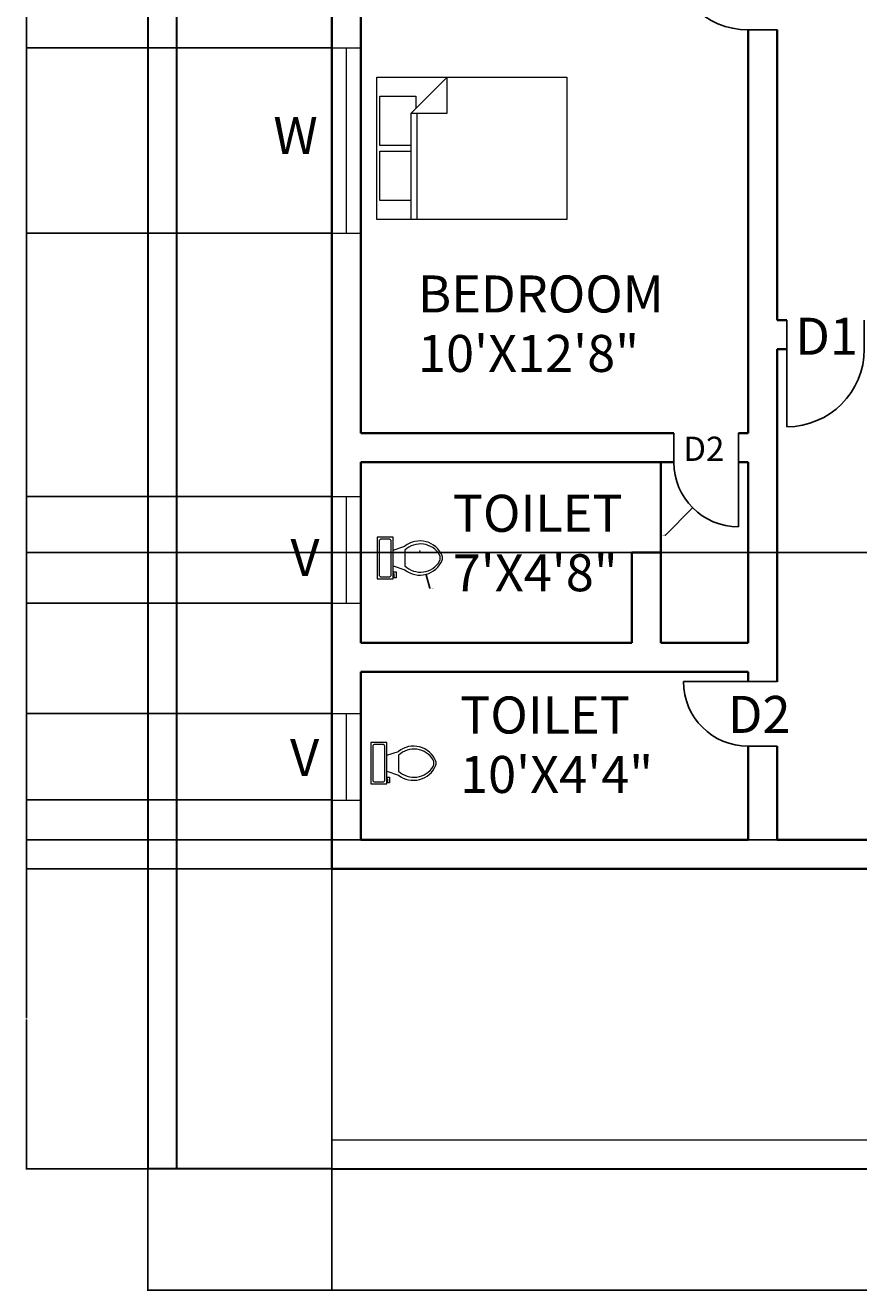
# Model space of a CAD drawing. Units: feet. Extents: x 1889 to 2708, y 1752 to 2375.
# Tile 1 of 5: x 1889 to 2147, y 1774 to 2166. Entities that reach past the tile are written whole.
import ezdxf

# ---------------------------------------------------------------- set-up
doc = ezdxf.new("R2010")
doc.units = ezdxf.units.FT
for name, color, linetype, lineweight in [('A-ANNO-DIMS', 2, 'Continuous', 18), ('A-ANNO-TEXT', 7, 'Continuous', 18), ('A-AREA-IDEN', 7, 'Continuous', 18), ('A-DOOR', 3, 'Continuous', 25), ('A-FLOR-FIXT', 8, 'Continuous', 18), ('A-FURN', 8, 'Continuous', 18), ('A-GLAZ', 4, 'Continuous', 18), ('A-WALL', 7, 'Continuous', 35), ('C-PROP', 7, 'Continuous', 30), ('C-SITE', 94, 'Continuous', 18)]:
    doc.layers.add(name, color=color, linetype=linetype, lineweight=lineweight)
doc.styles.get("Standard").update_dxf_attribs({"font": 'arial.ttf'})
doc.dimstyles.get("Standard").update_dxf_attribs({"dimtxt": 0.18, "dimasz": 0.18, "dimexe": 0.18, "dimexo": 0.0625, "dimgap": 0.09, "dimtad": 0, "dimtih": 1, "dimtoh": 1, "dimdec": 4, "dimzin": 0, "dimdsep": 46, "dimtxsty": 'Standard', "dimcen": 0.09, "dimadec": 0, "dimazin": 0, "dimtfac": 1, "dimtdec": 4, "dimtofl": 0, "dimtmove": 0, "dimatfit": 3, "dimfxl": 1, "dimtolj": 1, "dimtzin": 0, "dimarcsym": 0})

# ---------------------------------------------------------------- blocks, each defined once
blk = doc.blocks.new('Toilet - top')
for p, q in [((9.5, -6), (9.5, -2)), ((-10, -8.5), (-8, -8.5)), ((-10, -9.5), (-10, -8.5)), ((-7, -9.5), (-10, -9.5)), ((-8, -8.5), (-8, -8)), ((-7, -8), (-7, -9.5)), ((-4, -8), (-6, -14)), ((4, -8), (6, -14)), ((4, -14), (-4, -14))]:
    blk.add_line(p, q)
blk.add_lwpolyline([(10.5, -8), (10.5, 0), (-10.5, 0), (-10.5, -8)], close=True)
for points in [[(-9.5, -2), (-9.5, -6)], [(8.5, -1), (-8.5, -1)], [(-8.5, -7), (8.5, -7)]]:
    blk.add_lwpolyline(points)
for centre, radius, start, end in [((-8.62, -1.88), 0.884, 81.8699, 188.1301), ((-8.62, -6.12), 0.884, 171.8699, 278.1301), ((8.62, -1.88), 0.884, 351.8699, 98.1301), ((8.62, -6.12), 0.884, 261.8699, 8.1301), ((3.52, -21.58), 12.17, 141.46911, 247.97143), ((4.2, -21.82), 11.33, 136.36773, 238.94682), ((-3.52, -21.58), 12.17, 292.02843, 38.53071), ((-4.2, -21.82), 11.33, 301.05301, 43.63209), ((0, -27.88), 4, 245.73182, 294.26817), ((0, -29), 4, 254.86053, 285.13947)]:
    blk.add_arc(centre, radius, start, end)
blk = doc.blocks.new('Bed - Queen')
for p, q in [((0, -80.00003), (0, 0)), ((0, 0), (59.99999, 0)), ((59.99999, 0), (59.99999, -80.00003)), ((7.99999, -1.2), (28.79998, -1.2)), ((7.99999, -14.4), (7.99999, -1.2)), ((28.79998, -1.2), (28.79998, -14.4)), ((31.19999, -1.2), (51.99999, -1.2)), ((31.19999, -14.4), (31.19999, -1.2)), ((51.99999, -1.2), (51.99999, -16.4)), ((0, -14.4), (44.8, -14.4)), ((59.99999, -29.6), (44.8, -14.4)), ((44.8, -14.4), (44.8, -29.6)), ((44.8, -16.8), (0, -16.8)), ((51.99999, -16.4), (46.79936, -16.4)), ((44.8, -29.6), (59.99999, -29.6)), ((59.99999, -80.00003), (0, -80.00003))]:
    blk.add_line(p, q)
blk = doc.blocks.new('DOOR-SWING-24')
for p, q in [((9, 24), (0, 24)), ((33, 0), (0, 0))]:
    blk.add_line(p, q)
blk.add_arc((9, 0), 24, 0, 90)
blk = doc.blocks.new('DOOR-SWING-20')
for p, q in [((0, 29), (0, 0)), ((20, 9), (20, 0))]:
    blk.add_line(p, q)
blk.add_arc((0, 9), 20, 0, 90)
blk = doc.blocks.new('*D44')
at = {"layer": 'A-ANNO-DIMS', "color": 0, "lineweight": -2, "transparency": 16777216}
for p, q in [((1926.86, 1811.54), (1926.86, 1773.87)), ((2669.86, 1811.54), (2669.86, 1773.87)), ((1927.04, 1774.05), (2298.08, 1774.05)), ((2669.68, 1774.05), (2298.65, 1774.05))]:
    blk.add_line(p, q, dxfattribs=at)
at = {"layer": 'A-ANNO-DIMS', "color": 0, "transparency": 16777216}
for points in [[(1927.04, 1774.08), (1927.04, 1774.02), (1926.86, 1774.05)], [(2669.68, 1774.08), (2669.68, 1774.02), (2669.86, 1774.05)]]:
    blk.add_solid(points, dxfattribs=at)
at = {"layer": 'Defpoints', "color": 0, "transparency": 16777216}
for p in [(1926.86, 1811.6), (2669.86, 1811.6), (2669.86, 1774.05)]:
    blk.add_point(p, dxfattribs=at)
at = {"layer": 'A-ANNO-DIMS', "color": 0, "transparency": 16777216, "insert": (2298.36, 1774.05), "char_height": 0.18, "attachment_point": 5}
blk.add_mtext('\\A1;743', dxfattribs=at)
blk = doc.blocks.new('*D46')
at = {"layer": 'A-ANNO-DIMS', "color": 0, "lineweight": -2, "transparency": 16777216}
for p, q in [((1926.8, 2337.6), (1889.13, 2337.6)), ((1889.31, 2337.42), (1889.31, 2121.28)), ((1889.31, 1904.78), (1889.31, 2120.92)), ((1983.8, 1904.6), (1889.13, 1904.6))]:
    blk.add_line(p, q, dxfattribs=at)
at = {"layer": 'A-ANNO-DIMS', "color": 0, "transparency": 16777216}
for points in [[(1889.28, 2337.42), (1889.34, 2337.42), (1889.31, 2337.6)], [(1889.28, 1904.78), (1889.34, 1904.78), (1889.31, 1904.6)]]:
    blk.add_solid(points, dxfattribs=at)
at = {"layer": 'Defpoints', "color": 0, "transparency": 16777216}
for p in [(1889.31, 2337.6), (1926.86, 2337.6), (1983.86, 1904.6)]:
    blk.add_point(p, dxfattribs=at)
at = {"layer": 'A-ANNO-DIMS', "color": 0, "transparency": 16777216, "insert": (1889.31, 2121.1), "char_height": 0.18, "attachment_point": 5}
blk.add_mtext('\\A1;433', dxfattribs=at)
blk = doc.blocks.new('*D47')
at = {"layer": 'A-ANNO-DIMS', "color": 0, "lineweight": -2, "transparency": 16777216}
for p, q in [((1983.8, 1904.6), (1889.13, 1904.6)), ((1889.31, 1904.42), (1889.31, 1858.28)), ((1889.31, 1811.78), (1889.31, 1857.92)), ((1926.8, 1811.6), (1889.13, 1811.6))]:
    blk.add_line(p, q, dxfattribs=at)
at = {"layer": 'A-ANNO-DIMS', "color": 0, "transparency": 16777216}
for points in [[(1889.28, 1904.42), (1889.34, 1904.42), (1889.31, 1904.6)], [(1889.28, 1811.78), (1889.34, 1811.78), (1889.31, 1811.6)]]:
    blk.add_solid(points, dxfattribs=at)
at = {"layer": 'Defpoints', "color": 0, "transparency": 16777216}
for p in [(1889.31, 1904.6), (1983.86, 1904.6), (1926.86, 1811.6)]:
    blk.add_point(p, dxfattribs=at)
at = {"layer": 'A-ANNO-DIMS', "color": 0, "transparency": 16777216, "insert": (1889.31, 1858.1), "char_height": 0.18, "attachment_point": 5}
blk.add_mtext('\\A1;93', dxfattribs=at)
blk = doc.blocks.new('*D48')
at = {"layer": 'A-ANNO-DIMS', "color": 0, "lineweight": -2, "transparency": 16777216}
for p, q in [((1983.86, 1820.66), (1983.86, 2375.33)), ((1984.04, 2375.15), (2208.07, 2375.15)), ((2432.68, 2375.15), (2208.66, 2375.15)), ((2432.86, 1820.66), (2432.86, 2375.33))]:
    blk.add_line(p, q, dxfattribs=at)
at = {"layer": 'A-ANNO-DIMS', "color": 0, "transparency": 16777216}
for points in [[(1984.04, 2375.18), (1984.04, 2375.12), (1983.86, 2375.15)], [(2432.68, 2375.18), (2432.68, 2375.12), (2432.86, 2375.15)]]:
    blk.add_solid(points, dxfattribs=at)
at = {"layer": 'Defpoints', "color": 0, "transparency": 16777216}
for p in [(2432.86, 2375.15), (1983.86, 1820.6), (2432.86, 1820.6)]:
    blk.add_point(p, dxfattribs=at)
at = {"layer": 'A-ANNO-DIMS', "color": 0, "transparency": 16777216, "insert": (2208.36, 2375.15), "char_height": 0.18, "attachment_point": 5}
blk.add_mtext('\\A1;449', dxfattribs=at)
blk = doc.blocks.new('*D49')
at = {"layer": 'A-ANNO-DIMS', "color": 0, "lineweight": -2, "transparency": 16777216}
for p, q in [((1983.8, 1925.93), (1889.13, 1925.93)), ((1889.31, 1925.75), (1889.31, 1915.45)), ((1889.31, 1904.78), (1889.31, 1915.08)), ((1983.8, 1904.6), (1889.13, 1904.6))]:
    blk.add_line(p, q, dxfattribs=at)
at = {"layer": 'A-ANNO-DIMS', "color": 0, "transparency": 16777216}
for points in [[(1889.28, 1925.75), (1889.34, 1925.75), (1889.31, 1925.93)], [(1889.28, 1904.78), (1889.34, 1904.78), (1889.31, 1904.6)]]:
    blk.add_solid(points, dxfattribs=at)
at = {"layer": 'Defpoints', "color": 0, "transparency": 16777216}
for p in [(1889.31, 1925.93), (1983.86, 1925.93), (1983.86, 1904.6)]:
    blk.add_point(p, dxfattribs=at)
at = {"layer": 'A-ANNO-DIMS', "color": 0, "transparency": 16777216, "insert": (1889.31, 1915.26), "char_height": 0.18, "attachment_point": 5}
blk.add_mtext('\\A1;21.33', dxfattribs=at)
blk = doc.blocks.new('*D50')
at = {"layer": 'A-ANNO-DIMS', "color": 0, "lineweight": -2, "transparency": 16777216}
for p, q in [((1983.8, 1952.74), (1889.13, 1952.74)), ((1889.31, 1952.56), (1889.31, 1939.51)), ((1889.31, 1926.11), (1889.31, 1939.15)), ((1983.8, 1925.93), (1889.13, 1925.93))]:
    blk.add_line(p, q, dxfattribs=at)
at = {"layer": 'A-ANNO-DIMS', "color": 0, "transparency": 16777216}
for points in [[(1889.28, 1952.56), (1889.34, 1952.56), (1889.31, 1952.74)], [(1889.28, 1926.11), (1889.34, 1926.11), (1889.31, 1925.93)]]:
    blk.add_solid(points, dxfattribs=at)
at = {"layer": 'Defpoints', "color": 0, "transparency": 16777216}
for p in [(1889.31, 1952.74), (1983.86, 1952.74), (1983.86, 1925.93)]:
    blk.add_point(p, dxfattribs=at)
at = {"layer": 'A-ANNO-DIMS', "color": 0, "transparency": 16777216, "insert": (1889.31, 1939.33), "char_height": 0.18, "attachment_point": 5}
blk.add_mtext('\\A1;26.81', dxfattribs=at)
blk = doc.blocks.new('*D51')
at = {"layer": 'A-ANNO-DIMS', "color": 0, "lineweight": -2, "transparency": 16777216}
for p, q in [((1983.8, 1986.91), (1889.13, 1986.91)), ((1889.31, 1986.73), (1889.31, 1970.01)), ((1889.31, 1952.92), (1889.31, 1969.64)), ((1983.8, 1952.74), (1889.13, 1952.74))]:
    blk.add_line(p, q, dxfattribs=at)
at = {"layer": 'A-ANNO-DIMS', "color": 0, "transparency": 16777216}
for points in [[(1889.28, 1986.73), (1889.34, 1986.73), (1889.31, 1986.91)], [(1889.28, 1952.92), (1889.34, 1952.92), (1889.31, 1952.74)]]:
    blk.add_solid(points, dxfattribs=at)
at = {"layer": 'Defpoints', "color": 0, "transparency": 16777216}
for p in [(1889.31, 1986.91), (1983.86, 1986.91), (1983.86, 1952.74)]:
    blk.add_point(p, dxfattribs=at)
at = {"layer": 'A-ANNO-DIMS', "color": 0, "transparency": 16777216, "insert": (1889.31, 1969.83), "char_height": 0.18, "attachment_point": 5}
blk.add_mtext('\\A1;34.176', dxfattribs=at)
blk = doc.blocks.new('*D52')
at = {"layer": 'A-ANNO-DIMS', "color": 0, "lineweight": -2, "transparency": 16777216}
for p, q in [((1983.8, 2019.93), (1889.13, 2019.93)), ((1889.31, 2019.75), (1889.31, 2003.6)), ((1889.31, 1987.09), (1889.31, 2003.24)), ((1983.8, 1986.91), (1889.13, 1986.91))]:
    blk.add_line(p, q, dxfattribs=at)
at = {"layer": 'A-ANNO-DIMS', "color": 0, "transparency": 16777216}
for points in [[(1889.28, 2019.75), (1889.34, 2019.75), (1889.31, 2019.93)], [(1889.28, 1987.09), (1889.34, 1987.09), (1889.31, 1986.91)]]:
    blk.add_solid(points, dxfattribs=at)
at = {"layer": 'Defpoints', "color": 0, "transparency": 16777216}
for p in [(1889.31, 2019.93), (1983.86, 2019.93), (1983.86, 1986.91)]:
    blk.add_point(p, dxfattribs=at)
at = {"layer": 'A-ANNO-DIMS', "color": 0, "transparency": 16777216, "insert": (1889.31, 2003.42), "char_height": 0.18, "attachment_point": 5}
blk.add_mtext('\\A1;33.02', dxfattribs=at)
blk = doc.blocks.new('*D53')
at = {"layer": 'A-ANNO-DIMS', "color": 0, "lineweight": -2, "transparency": 16777216}
for p, q in [((1983.8, 2101.58), (1889.13, 2101.58)), ((1889.31, 2101.4), (1889.31, 2060.94)), ((1889.31, 2020.11), (1889.31, 2060.57)), ((1983.8, 2019.93), (1889.13, 2019.93))]:
    blk.add_line(p, q, dxfattribs=at)
at = {"layer": 'A-ANNO-DIMS', "color": 0, "transparency": 16777216}
for points in [[(1889.28, 2101.4), (1889.34, 2101.4), (1889.31, 2101.58)], [(1889.28, 2020.11), (1889.34, 2020.11), (1889.31, 2019.93)]]:
    blk.add_solid(points, dxfattribs=at)
at = {"layer": 'Defpoints', "color": 0, "transparency": 16777216}
for p in [(1889.31, 2101.58), (1983.86, 2101.58), (1983.86, 2019.93)]:
    blk.add_point(p, dxfattribs=at)
at = {"layer": 'A-ANNO-DIMS', "color": 0, "transparency": 16777216, "insert": (1889.31, 2060.76), "char_height": 0.18, "attachment_point": 5}
blk.add_mtext('\\A1;81.65', dxfattribs=at)
blk = doc.blocks.new('*D54')
at = {"layer": 'A-ANNO-DIMS', "color": 0, "lineweight": -2, "transparency": 16777216}
for p, q in [((1983.8, 2159), (1889.13, 2159)), ((1889.31, 2158.82), (1889.31, 2130.47)), ((1889.31, 2101.76), (1889.31, 2130.11)), ((1983.8, 2101.58), (1889.13, 2101.58))]:
    blk.add_line(p, q, dxfattribs=at)
at = {"layer": 'A-ANNO-DIMS', "color": 0, "transparency": 16777216}
for points in [[(1889.28, 2158.82), (1889.34, 2158.82), (1889.31, 2159)], [(1889.28, 2101.76), (1889.34, 2101.76), (1889.31, 2101.58)]]:
    blk.add_solid(points, dxfattribs=at)
at = {"layer": 'Defpoints', "color": 0, "transparency": 16777216}
for p in [(1889.31, 2159), (1983.86, 2159), (1983.86, 2101.58)]:
    blk.add_point(p, dxfattribs=at)
at = {"layer": 'A-ANNO-DIMS', "color": 0, "transparency": 16777216, "insert": (1889.31, 2130.29), "char_height": 0.18, "attachment_point": 5}
blk.add_mtext('\\A1;57.41', dxfattribs=at)
blk = doc.blocks.new('*D55')
at = {"layer": 'A-ANNO-DIMS', "color": 0, "lineweight": -2, "transparency": 16777216}
for p, q in [((1983.8, 2203.6), (1889.13, 2203.6)), ((1889.31, 2203.42), (1889.31, 2181.48)), ((1889.31, 2159.18), (1889.31, 2181.12)), ((1983.8, 2159), (1889.13, 2159))]:
    blk.add_line(p, q, dxfattribs=at)
at = {"layer": 'A-ANNO-DIMS', "color": 0, "transparency": 16777216}
for points in [[(1889.28, 2203.42), (1889.34, 2203.42), (1889.31, 2203.6)], [(1889.28, 2159.18), (1889.34, 2159.18), (1889.31, 2159)]]:
    blk.add_solid(points, dxfattribs=at)
at = {"layer": 'Defpoints', "color": 0, "transparency": 16777216}
for p in [(1889.31, 2203.6), (1983.86, 2203.6), (1983.86, 2159)]:
    blk.add_point(p, dxfattribs=at)
at = {"layer": 'A-ANNO-DIMS', "color": 0, "transparency": 16777216, "insert": (1889.31, 2181.3), "char_height": 0.18, "attachment_point": 5}
blk.add_mtext('\\A1;44.6', dxfattribs=at)
blk = doc.blocks.new('*D58')
at = {"layer": 'A-ANNO-DIMS', "color": 0, "lineweight": -2, "transparency": 16777216}
for p, q in [((1983.86, 1904.54), (1983.86, 1773.87)), ((2159.47, 1904.54), (2159.47, 1773.87)), ((1984.04, 1774.05), (2071.28, 1774.05)), ((2159.29, 1774.05), (2072.05, 1774.05))]:
    blk.add_line(p, q, dxfattribs=at)
at = {"layer": 'A-ANNO-DIMS', "color": 0, "transparency": 16777216}
for points in [[(1984.04, 1774.08), (1984.04, 1774.02), (1983.86, 1774.05)], [(2159.29, 1774.08), (2159.29, 1774.02), (2159.47, 1774.05)]]:
    blk.add_solid(points, dxfattribs=at)
at = {"layer": 'Defpoints', "color": 0, "transparency": 16777216}
for p in [(1983.86, 1904.6), (2159.47, 1904.6), (2159.47, 1774.05)]:
    blk.add_point(p, dxfattribs=at)
at = {"layer": 'A-ANNO-DIMS', "color": 0, "transparency": 16777216, "insert": (2071.67, 1774.05), "char_height": 0.18, "attachment_point": 5}
blk.add_mtext('\\A1;175.6', dxfattribs=at)
blk = doc.blocks.new('*D60')
at = {"layer": 'A-ANNO-DIMS', "color": 0, "lineweight": -2, "transparency": 16777216}
for p, q in [((2423.8, 2002.6), (1889.13, 2002.6)), ((1889.31, 2002.42), (1889.31, 1958.28)), ((1889.31, 1913.78), (1889.31, 1957.92)), ((2423.8, 1913.6), (1889.13, 1913.6))]:
    blk.add_line(p, q, dxfattribs=at)
at = {"layer": 'A-ANNO-DIMS', "color": 0, "transparency": 16777216}
for points in [[(1889.28, 2002.42), (1889.34, 2002.42), (1889.31, 2002.6)], [(1889.28, 1913.78), (1889.34, 1913.78), (1889.31, 1913.6)]]:
    blk.add_solid(points, dxfattribs=at)
at = {"layer": 'Defpoints', "color": 0, "transparency": 16777216}
for p in [(1889.31, 2002.6), (2423.86, 2002.6), (2423.86, 1913.6)]:
    blk.add_point(p, dxfattribs=at)
at = {"layer": 'A-ANNO-DIMS', "color": 0, "transparency": 16777216, "insert": (1889.31, 1958.1), "char_height": 0.18, "attachment_point": 5}
blk.add_mtext('\\A1;89', dxfattribs=at)
blk = doc.blocks.new('*D66')
at = {"layer": 'A-ANNO-DIMS', "color": 0, "lineweight": -2, "transparency": 16777216}
for p, q in [((2109.77, 2030.6), (2109.95, 2030.6)), ((2109.86, 2030.51), (2109.86, 2030.69)), ((2087.24, 2007.97), (2095.59, 2016.33)), ((2087.06, 2007.97), (2087.24, 2007.97))]:
    blk.add_line(p, q, dxfattribs=at)
at = {"layer": 'A-ANNO-DIMS', "color": 0, "transparency": 16777216}
blk.add_solid([(2095.57, 2016.35), (2095.62, 2016.31), (2095.72, 2016.46)], dxfattribs=at)
at = {"layer": 'Defpoints', "color": 0, "transparency": 16777216}
for p in [(2109.86, 2030.6), (2095.72, 2016.46)]:
    blk.add_point(p, dxfattribs=at)
at = {"layer": 'A-ANNO-DIMS', "color": 0, "transparency": 16777216, "insert": (2086.56, 2007.97), "char_height": 0.18, "attachment_point": 5}
blk.add_mtext('\\A1;2X R20', dxfattribs=at)
blk = doc.blocks.new('*D71')
at = {"layer": 'A-ANNO-DIMS', "color": 0, "lineweight": -2, "transparency": 16777216}
for p, q in [((2011.11, 2003.08), (2011.29, 2003.08)), ((2011.2, 2002.99), (2011.2, 2003.17)), ((2014.23, 1991.54), (2013.14, 1995.69)), ((2014.41, 1991.54), (2014.23, 1991.54))]:
    blk.add_line(p, q, dxfattribs=at)
at = {"layer": 'A-ANNO-DIMS', "color": 0, "transparency": 16777216}
blk.add_solid([(2013.17, 1995.7), (2013.11, 1995.68), (2013.09, 1995.87)], dxfattribs=at)
at = {"layer": 'Defpoints', "color": 0, "transparency": 16777216}
for p in [(2011.2, 2003.08), (2013.09, 1995.87)]:
    blk.add_point(p, dxfattribs=at)
at = {"layer": 'A-ANNO-DIMS', "color": 0, "transparency": 16777216, "insert": (2015.08, 1991.54), "char_height": 0.18, "attachment_point": 5}
blk.add_mtext('\\A1;6X R7.455', dxfattribs=at)

msp = doc.modelspace()

# ---------------------------------------------------------------- linework, layer by layer
at = {"layer": 'A-GLAZ'}
for p, q in [((1983.8644, 2158.9974), (1992.8644, 2158.9974)), ((1988.3644, 2158.9974), (1988.3644, 2101.5825)), ((1983.8644, 2101.5825), (1992.8644, 2101.5825)), ((1983.8644, 2019.9308), (1992.8644, 2019.9308)), ((1988.3644, 2019.9308), (1988.3644, 1986.9135)), ((1983.8644, 1986.9135), (1992.8644, 1986.9135)), ((1983.8644, 1952.7379), (1992.8644, 1952.7379)), ((1988.3644, 1952.7379), (1988.3644, 1925.928)), ((1983.8644, 1925.928), (1992.8644, 1925.928))]:
    msp.add_line(p, q, dxfattribs=at)
at = {"layer": 'A-WALL'}
for p, q in [((1983.8644, 2203.5988), (1983.8644, 1904.5988)), ((1983.8644, 2203.5988), (1983.8644, 1974.5988)), ((1983.8644, 2203.5988), (1983.8644, 2039.5988)), ((1992.8644, 2191.5988), (1992.8644, 2039.5988)), ((2112.8644, 2039.5988), (2112.8644, 2164.5988)), ((2121.8644, 2074.5988), (2121.8644, 2164.5988)), ((2121.8644, 2164.5988), (2121.8644, 2074.5988)), ((2121.8644, 2074.5988), (2124.8644, 2074.5988)), ((2121.8644, 2039.5988), (2121.8644, 2065.5988)), ((2121.8644, 2065.5988), (2124.8644, 2065.5988)), ((2121.8644, 2065.5988), (2121.8644, 1962.5988)), ((1992.8644, 2039.5988), (2089.8644, 2039.5988)), ((2109.8644, 2039.5988), (2112.8644, 2039.5988)), ((1992.8644, 2030.5988), (2085.8644, 2030.5988)), ((1992.8644, 2030.5988), (1992.8644, 1974.5988)), ((2085.8644, 1974.5988), (2085.8644, 2030.5988)), ((2085.8644, 2030.5988), (2089.8644, 2030.5988)), ((2109.8644, 2030.5988), (2112.8644, 2030.5988)), ((2112.8644, 2030.5988), (2112.8644, 1974.5988)), ((2121.8644, 2030.5988), (2121.8644, 1974.5988)), ((2076.8644, 1974.5988), (2076.8644, 2002.5988)), ((2085.8644, 2002.5988), (2076.8644, 2002.5988)), ((1992.8644, 1974.5988), (2076.8644, 1974.5988)), ((2085.8644, 1974.5988), (2112.8644, 1974.5988)), ((1992.8644, 1965.5988), (2076.8644, 1965.5988)), ((1992.8644, 1965.5988), (2112.8644, 1965.5988)), ((1992.8644, 1965.5988), (1992.8644, 1913.5988)), ((2112.8644, 1962.5988), (2112.8644, 1965.5988)), ((2121.8644, 1962.5988), (2121.8644, 1965.5988)), ((2112.8644, 1913.5988), (2112.8644, 1942.5988)), ((2121.8644, 1913.5988), (2121.8644, 1942.5988)), ((2121.8644, 1942.5988), (2121.8644, 1913.5988)), ((1992.8644, 1913.5988), (2112.8644, 1913.5988)), ((2121.8644, 1913.5988), (2270.8644, 1913.5988)), ((1983.8644, 1904.5988), (2112.8644, 1904.5988)), ((2112.8644, 1904.5988), (2121.8644, 1904.5988)), ((2121.8644, 1904.5988), (2432.8644, 1904.5988))]:
    msp.add_line(p, q, dxfattribs=at)
at = {"layer": 'C-PROP'}
for p, q in [((1935.8644, 1811.5988), (1935.8644, 2328.5988)), ((1926.8644, 2236.5988), (1926.8644, 1811.5988)), ((1983.8644, 1811.5988), (1926.8644, 1811.5988)), ((1983.8644, 1811.5988), (2432.8644, 1811.5988))]:
    msp.add_line(p, q, dxfattribs=at)
at = {"layer": 'C-SITE'}
for p, q in [((1983.8644, 1904.5988), (1983.8644, 1811.5988)), ((1983.8644, 1820.5988), (2432.8644, 1820.5988))]:
    msp.add_line(p, q, dxfattribs=at)

# ---------------------------------------------------------------- block references
at = {"layer": 'A-DOOR'}
for name, p, rotation in [('DOOR-SWING-24', (2121.8649, 2188.5986), 180), ('DOOR-SWING-24', (2124.8647, 2074.5992), 269.9999999999978), ('DOOR-SWING-20', (2109.8649, 2039.5986), 180)]:
    msp.add_blockref(name, p, dxfattribs=dict(at, rotation=rotation))
at = {"layer": 'A-DOOR', "extrusion": (0, 0, -1), "zscale": -1, "rotation": 270.0000000000031}
msp.add_blockref('DOOR-SWING-20', (-2121.8642, 1962.5992), dxfattribs=at)
at = {"layer": 'A-FLOR-FIXT', "xscale": 0.6125984407344605, "yscale": 0.6125984407344605, "zscale": 0.6125984407344605, "rotation": 90}
for p in [(1997.9777, 2000.9195), (1995.9966, 1937.3276)]:
    msp.add_blockref('Toilet - top', p, dxfattribs=at)
at = {"layer": 'A-FURN', "xscale": 0.7363101783767424, "yscale": 0.7363101783767424, "zscale": 0.7363101783767424, "rotation": 90}
msp.add_blockref('Bed - Queen', (1997.8426, 2105.7821), dxfattribs=at)

# ---------------------------------------------------------------- texts
at = {"layer": 'A-ANNO-TEXT'}
for s, height, p in [('W', 11.4692, (1965.793, 2126.0917)), ('D1', 11.46921, (2127.4546, 2063.9019)), ('D2', 7.52883, (2092.7652, 2030.9991)), ('V', 11.4692, (1971.0925, 1995.3498)), ('D2', 11.46921, (2106.5688, 1946.7115)), ('V', 11.4692, (1970.9619, 1933.349))]:
    msp.add_text(s, height=height, dxfattribs=at).set_placement(p)
at = {"layer": 'A-AREA-IDEN'}
for s, p in [('BEDROOM', (2010.6091, 2077.0075)), ('10\'X12\'8"', (2010.6091, 2058.5832)), ('TOILET', (2021.3596, 2009.0396)), ('7\'X4\'8"', (2021.3596, 1990.6153)), ('TOILET', (2023.6355, 1946.534)), ('10\'X4\'4"', (2023.6355, 1928.1097))]:
    msp.add_text(s, height=11.46921, dxfattribs=at).set_placement(p)

# ---------------------------------------------------------------- dimensions: what is measured, and where the dimension line sits
at = {"layer": 'A-ANNO-DIMS'}
for base, p1, p2, override, picture, middle in [((2432.8644, 2375.1488), (1983.8644, 1820.5988), (2432.8644, 1820.5988), {"dimdec": 0, "dimlfac": 1, "dimrnd": 0, "dimzin": 0, "dimdsep": 46, "dimlunit": 2}, '*D48', (2208.3644, 2375.1488)), ((2159.4686, 1774.0488), (1983.8644, 1904.5988), (2159.4686, 1904.5988), {"dimdec": 1, "dimlfac": 1, "dimrnd": 0, "dimzin": 0, "dimdsep": 46, "dimlunit": 2}, '*D58', (2071.6665, 1774.0488)), ((2669.8644, 1774.0488), (1926.8644, 1811.5988), (2669.8644, 1811.5988), {"dimdec": 0, "dimlfac": 1, "dimrnd": 0, "dimzin": 0, "dimdsep": 46, "dimlunit": 2}, '*D44', (2298.3644, 1774.0488))]:
    dim = msp.add_linear_dim(base=base, p1=p1, p2=p2, dimstyle='Standard', override=override, dxfattribs=at)
    dim.commit()
    dim.dimension.update_dxf_attribs({"geometry": picture, "text_midpoint": middle})
for base, p1, p2, override, picture, middle in [((1889.3144, 2337.5988), (1983.8644, 1904.5988), (1926.8644, 2337.5988), {"dimdec": 0, "dimlfac": 1, "dimrnd": 0, "dimzin": 0, "dimdsep": 46, "dimlunit": 2}, '*D46', (1889.3144, 2121.0988)), ((1889.3144, 2203.5988), (1983.8644, 2158.9974), (1983.8644, 2203.5988), {"dimdec": 1, "dimlfac": 1, "dimrnd": 0, "dimzin": 0, "dimdsep": 46, "dimlunit": 2}, '*D55', (1889.3144, 2181.2981)), ((1889.3144, 2158.9974), (1983.8644, 2101.5825), (1983.8644, 2158.9974), {"dimdec": 2, "dimlfac": 1, "dimrnd": 0, "dimzin": 0, "dimdsep": 46, "dimlunit": 2}, '*D54', (1889.3144, 2130.2899)), ((1889.3144, 2101.5825), (1983.8644, 2019.9308), (1983.8644, 2101.5825), {"dimdec": 2, "dimlfac": 1, "dimrnd": 0, "dimzin": 0, "dimdsep": 46, "dimlunit": 2}, '*D53', (1889.3144, 2060.7566)), ((1889.3144, 2019.9308), (1983.8644, 1986.9135), (1983.8644, 2019.9308), {"dimdec": 2, "dimlfac": 1, "dimrnd": 0, "dimzin": 0, "dimdsep": 46, "dimlunit": 2}, '*D52', (1889.3144, 2003.4222)), ((1889.3144, 2002.5988), (2423.8644, 1913.5988), (2423.8644, 2002.5988), {"dimdec": 0, "dimlfac": 1, "dimrnd": 0, "dimzin": 0, "dimdsep": 46, "dimlunit": 2}, '*D60', (1889.3144, 1958.0988)), ((1889.3144, 1986.9135), (1983.8644, 1952.7379), (1983.8644, 1986.9135), {"dimdec": 3, "dimlfac": 1, "dimrnd": 0, "dimzin": 0, "dimdsep": 46, "dimlunit": 2}, '*D51', (1889.3144, 1969.8257)), ((1889.3144, 1952.7379), (1983.8644, 1925.928), (1983.8644, 1952.7379), {"dimdec": 2, "dimlfac": 1, "dimrnd": 0, "dimzin": 0, "dimdsep": 46, "dimlunit": 2}, '*D50', (1889.3144, 1939.3329)), ((1889.3144, 1925.928), (1983.8644, 1904.5988), (1983.8644, 1925.928), {"dimdec": 2, "dimlfac": 1, "dimrnd": 0, "dimzin": 0, "dimdsep": 46, "dimlunit": 2}, '*D49', (1889.3144, 1915.2634)), ((1889.3144, 1904.5988), (1926.8644, 1811.5988), (1983.8644, 1904.5988), {"dimdec": 0, "dimlfac": 1, "dimrnd": 0, "dimzin": 0, "dimdsep": 46, "dimlunit": 2}, '*D47', (1889.3144, 1858.0988))]:
    dim = msp.add_linear_dim(base=base, p1=p1, p2=p2, angle=90, dimstyle='Standard', override=override, dxfattribs=at)
    dim.commit()
    dim.dimension.update_dxf_attribs({"geometry": picture, "text_midpoint": middle})
for center, mpoint, text, override, picture, middle in [((2109.8644, 2030.5988), (2095.722, 2016.457), '2X <>', {"dimdec": 0, "dimlfac": 1, "dimrnd": 0, "dimzin": 0, "dimdsep": 46, "dimlunit": 2}, '*D66', (2086.5568, 2007.9719)), ((2011.1979, 2003.0756), (2013.0921, 1995.8655), '6X <>', {"dimdec": 3, "dimlfac": 1, "dimrnd": 0, "dimzin": 0, "dimdsep": 46, "dimlunit": 2}, '*D71', (2015.0831, 1991.5395))]:
    dim = msp.add_radius_dim(center=center, mpoint=mpoint, text=text, dimstyle='Standard', override=override, dxfattribs=at)
    dim.commit()
    dim.dimension.update_dxf_attribs({"geometry": picture, "text_midpoint": middle, "dimtype": 164})

doc.saveas('drawing.dxf')
